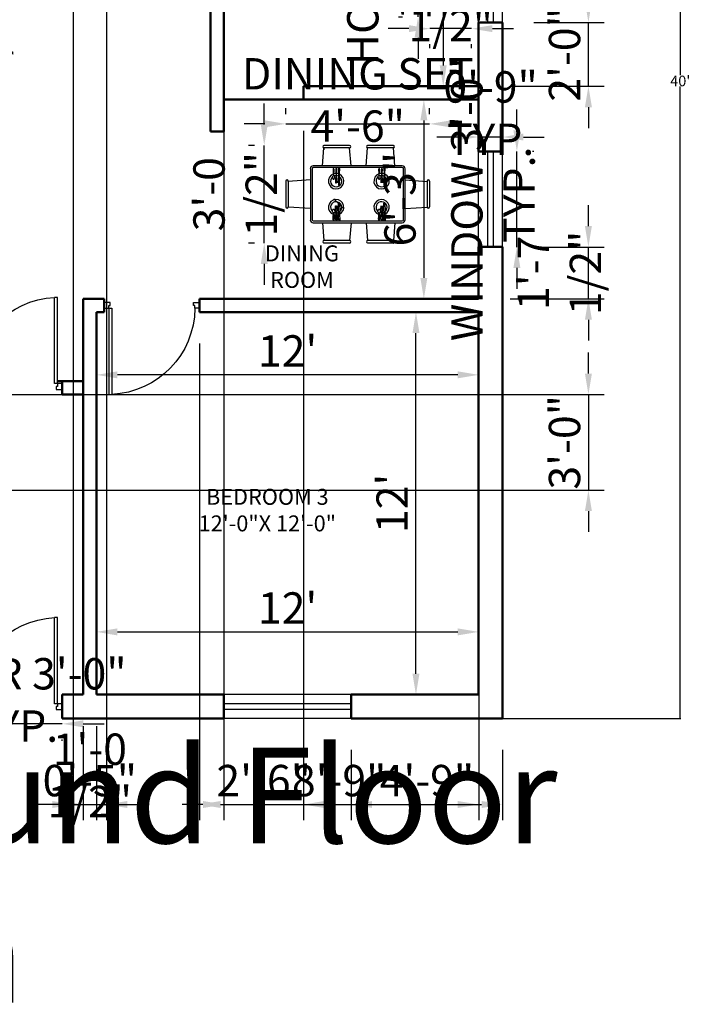
# Model space of a CAD drawing. Units: inches. Extents: x 117606 to 118050, y 251709 to 252357.
# Tile 2 of 3: x 117797 to 118050, y 251709 to 252079. Entities that reach past the tile are written whole.
import ezdxf

# ---------------------------------------------------------------- set-up
doc = ezdxf.new("R2010")
doc.units = ezdxf.units.IN
doc.header["$MEASUREMENT"] = 0
doc.layers.add('a patt', color=33, linetype='Continuous')
for name, color, linetype, lineweight in [('A-ANNO-TEXT', 7, 'Continuous', 25), ('A-AREA-IDEN', 7, 'Continuous', 25), ('A-DOOR', 4, 'Continuous', 25), ('FURNITURE', 53, 'Continuous', 18), ('WALL', 7, 'Continuous', 50), ('WINDOW', 2, 'Continuous', 25), ('YQ_DIM', 3, 'Continuous', 18)]:
    doc.layers.add(name, color=color, linetype=linetype, lineweight=lineweight)
doc.styles.get("Standard").update_dxf_attribs({"font": 'arial.ttf'})
doc.styles.add('YQ_DIM', font='SUPEROS.SHX', dxfattribs={"width": 0.8, "bigfont": 'HZDX.SHX'})
doc.dimstyles.get("Standard").update_dxf_attribs({"dimtxt": 4, "dimasz": 0.18, "dimexe": 0.18, "dimexo": 0.0625, "dimgap": 0.09, "dimtad": 0, "dimtih": 1, "dimtoh": 1, "dimzin": 0, "dimdsep": 46, "dimlunit": 4, "dimtxsty": 'Standard', "dimcen": 0.09, "dimadec": 0, "dimazin": 0, "dimtfac": 1, "dimtofl": 0, "dimtmove": 0, "dimatfit": 3, "dimfxl": 1, "dimtolj": 1, "dimtzin": 0, "dimarcsym": 0})
doc.dimstyles.new('yqi3_937', dxfattribs={"dimscale": 3.937008, "dimtxt": 3, "dimasz": 2, "dimexe": 1.5, "dimexo": 3, "dimgap": 0.5, "dimtad": 1, "dimdsep": 46, "dimlunit": 4, "dimtxsty": 'YQ_DIM', "dimcen": 0, "dimclrd": 256, "dimclre": 256, "dimclrt": 7, "dimadec": 1, "dimazin": 2, "dimtfac": 1, "dimtix": 1, "dimtmove": 2, "dimatfit": 2, "dimfxl": 1, "dimtolj": 1, "dimtzin": 0, "dimarcsym": 0})

# ---------------------------------------------------------------- blocks, each defined once
blk = doc.blocks.new('*D2')
at = {"layer": 'Defpoints', "color": 0, "transparency": 16777216}
for p in [(117978.89, 252296.28), (117978.89, 251816.28), (118045.85, 251816.28)]:
    blk.add_point(p, dxfattribs=at)
at = {"layer": 'YQ_DIM', "color": 0, "lineweight": -2, "transparency": 16777216}
for p, q in [((117978.95, 252296.28), (118046.03, 252296.28)), ((118045.85, 252296.1), (118045.85, 252058.42)), ((118045.85, 251816.46), (118045.85, 252054.15)), ((117978.95, 251816.28), (118046.03, 251816.28))]:
    blk.add_line(p, q, dxfattribs=at)
at = {"layer": 'YQ_DIM', "color": 0, "transparency": 16777216}
for points in [[(118045.82, 252296.1), (118045.88, 252296.1), (118045.85, 252296.28)], [(118045.82, 251816.46), (118045.88, 251816.46), (118045.85, 251816.28)]]:
    blk.add_solid(points, dxfattribs=at)
at = {"layer": 'YQ_DIM', "color": 0, "transparency": 16777216, "insert": (118045.85, 252056.28), "char_height": 4, "attachment_point": 5}
blk.add_mtext("\\A1;40'", dxfattribs=at)
blk = doc.blocks.new('*D6')
at = {"layer": 'Defpoints', "color": 0, "transparency": 16777216}
for p in [(117825.89, 251969.28), (117969.89, 251969.28), (117825.89, 251945.66)]:
    blk.add_point(p, dxfattribs=at)
at = {"layer": 'YQ_DIM', "color": 0, "lineweight": -2, "transparency": 16777216}
for p, q in [((117825.89, 251957.47), (117825.89, 251939.76)), ((117969.89, 251957.47), (117969.89, 251939.76)), ((117962.01, 251945.66), (117833.76, 251945.66))]:
    blk.add_line(p, q, dxfattribs=at)
at = {"layer": 'YQ_DIM', "color": 0, "transparency": 16777216}
for points in [[(117833.76, 251946.97), (117833.76, 251944.35), (117825.89, 251945.66)], [(117962.01, 251946.97), (117962.01, 251944.35), (117969.89, 251945.66)]]:
    blk.add_solid(points, dxfattribs=at)
at = {"layer": 'YQ_DIM', "color": 0, "transparency": 16777216, "insert": (117897.89, 251954.66), "char_height": 11.811, "attachment_point": 5, "style": 'YQ_DIM'}
blk.add_mtext("\\A1;12'", dxfattribs=at)
blk = doc.blocks.new('*D7')
at = {"layer": 'Defpoints', "color": 0, "transparency": 16777216}
for p in [(117969.89, 251848.91), (117825.89, 251825.28), (117969.89, 251825.28)]:
    blk.add_point(p, dxfattribs=at)
at = {"layer": 'YQ_DIM', "color": 0, "lineweight": -2, "transparency": 16777216}
for p, q in [((117825.89, 251837.1), (117825.89, 251854.81)), ((117969.89, 251837.1), (117969.89, 251854.81)), ((117833.76, 251848.91), (117962.01, 251848.91))]:
    blk.add_line(p, q, dxfattribs=at)
at = {"layer": 'YQ_DIM', "color": 0, "transparency": 16777216}
for points in [[(117833.76, 251850.22), (117833.76, 251847.59), (117825.89, 251848.91)], [(117962.01, 251850.22), (117962.01, 251847.59), (117969.89, 251848.91)]]:
    blk.add_solid(points, dxfattribs=at)
at = {"layer": 'YQ_DIM', "color": 0, "transparency": 16777216, "insert": (117897.89, 251857.9), "char_height": 11.811, "attachment_point": 5, "style": 'YQ_DIM'}
blk.add_mtext("\\A1;12'", dxfattribs=at)
blk = doc.blocks.new('*D8')
at = {"layer": 'Defpoints', "color": 0, "transparency": 16777216}
for p in [(117946.26, 251969.28), (117969.89, 251969.28), (117969.89, 251825.28)]:
    blk.add_point(p, dxfattribs=at)
at = {"layer": 'YQ_DIM', "color": 0, "lineweight": -2, "transparency": 16777216}
for p, q in [((117958.07, 251969.28), (117940.36, 251969.28)), ((117946.26, 251833.16), (117946.26, 251961.41)), ((117958.07, 251825.28), (117940.36, 251825.28))]:
    blk.add_line(p, q, dxfattribs=at)
at = {"layer": 'YQ_DIM', "color": 0, "transparency": 16777216}
for points in [[(117944.95, 251961.41), (117947.58, 251961.41), (117946.26, 251969.28)], [(117944.95, 251833.16), (117947.58, 251833.16), (117946.26, 251825.28)]]:
    blk.add_solid(points, dxfattribs=at)
at = {"layer": 'YQ_DIM', "color": 0, "transparency": 16777216, "insert": (117937.26, 251897.28), "char_height": 11.811, "attachment_point": 5, "rotation": 90, "style": 'YQ_DIM'}
blk.add_mtext("\\A1;12'", dxfattribs=at)
blk = doc.blocks.new('*D9')
at = {"layer": 'Defpoints', "color": 0, "transparency": 16777216}
for p in [(117969.89, 252138.28), (117956.53, 252054.28), (117969.89, 252054.28)]:
    blk.add_point(p, dxfattribs=at)
at = {"layer": 'YQ_DIM', "color": 0, "lineweight": -2, "transparency": 16777216}
for p, q in [((117958.07, 252138.28), (117950.63, 252138.28)), ((117956.53, 252130.41), (117956.53, 252062.16)), ((117958.07, 252054.28), (117950.63, 252054.28))]:
    blk.add_line(p, q, dxfattribs=at)
at = {"layer": 'YQ_DIM', "color": 0, "transparency": 16777216}
for points in [[(117955.22, 252130.41), (117957.84, 252130.41), (117956.53, 252138.28)], [(117955.22, 252062.16), (117957.84, 252062.16), (117956.53, 252054.28)]]:
    blk.add_solid(points, dxfattribs=at)
at = {"layer": 'YQ_DIM', "color": 0, "transparency": 16777216, "insert": (117947.53, 252096.28), "char_height": 11.811, "attachment_point": 5, "rotation": 90, "style": 'YQ_DIM'}
blk.add_mtext("\\A1;7'", dxfattribs=at)
blk = doc.blocks.new('*D10')
at = {"layer": 'Defpoints', "color": 0, "transparency": 16777216}
for p in [(117969.89, 252049.28), (117949.24, 251974.28), (117969.89, 251974.28)]:
    blk.add_point(p, dxfattribs=at)
at = {"layer": 'YQ_DIM', "color": 0, "lineweight": -2, "transparency": 16777216}
for p, q in [((117958.07, 252049.28), (117943.34, 252049.28)), ((117949.24, 252041.41), (117949.24, 251982.16)), ((117958.07, 251974.28), (117943.34, 251974.28))]:
    blk.add_line(p, q, dxfattribs=at)
at = {"layer": 'YQ_DIM', "color": 0, "transparency": 16777216}
for points in [[(117947.93, 252041.41), (117950.55, 252041.41), (117949.24, 252049.28)], [(117947.93, 251982.16), (117950.55, 251982.16), (117949.24, 251974.28)]]:
    blk.add_solid(points, dxfattribs=at)
at = {"layer": 'YQ_DIM', "color": 0, "transparency": 16777216, "insert": (117940.24, 252011.78), "char_height": 11.811, "attachment_point": 5, "rotation": 90, "style": 'YQ_DIM'}
blk.add_mtext('\\A1;6\'-3"', dxfattribs=at)
blk = doc.blocks.new('DR_D01')
for p, q in [((-0.45, 0.93), (-0.42, 0.93)), ((-0.45, 0.03), (-0.45, 0.93)), ((-0.42, 0.03), (-0.42, 0.93)), ((-0.5, 0.03), (-0.42, 0.03)), ((-0.5, 0.03), (-0.5, -0.03)), ((-0.45, 0.03), (-0.45, 0)), ((-0.45, 0), (-0.435, 0)), ((-0.435, 0), (-0.435, -0.03)), ((0.435, 0), (0.435, -0.03)), ((0.45, 0), (0.435, 0)), ((0.45, 0.03), (0.45, 0)), ((0.5, 0.03), (0.45, 0.03)), ((0.5, -0.03), (0.5, 0.03)), ((-0.435, -0.03), (-0.5, -0.03)), ((0.435, -0.03), (0.5, -0.03))]:
    blk.add_line(p, q)
blk.add_arc((-0.46, 0.021), 0.91, 0.5915, 87.4664)
blk = doc.blocks.new('WD_WIN4')
for p, q in [((-0.5, 0.5), (0.5, 0.5)), ((-0.5, 0.12), (0.5, 0.12)), ((-0.5, -0.12), (0.5, -0.12)), ((-0.5, -0.5), (0.5, -0.5))]:
    blk.add_line(p, q)
blk = doc.blocks.new('grdfg')
at = {"layer": 'a patt'}
for p, q in [((30493, 21433), (30516, 21715)), ((30514, 21715), (30514, 21683)), ((30519, 21754), (30516, 21754)), ((30923, 21715), (30516, 21715)), ((30920, 21754), (30519, 21754)), ((30519, 21754), (30519, 21754)), ((30920, 21754), (30923, 21754)), ((30946, 21433), (30923, 21715)), ((31186, 21433), (31208, 21715)), ((31615, 21715), (31208, 21715)), ((31212, 21754), (31209, 21754)), ((31212, 21754), (31212, 21754)), ((31612, 21754), (31212, 21754)), ((31612, 21754), (31615, 21754)), ((31638, 21433), (31615, 21715)), ((30509, 21606), (30507, 21606)), ((31202, 21606), (31200, 21606)), ((30302, 21386), (30302, 20580)), ((30329, 21386), (30329, 20580)), ((31755, 21433), (30348, 21433)), ((31755, 21405), (30348, 21405)), ((30745, 21374), (30767, 21374)), ((31464, 21374), (31486, 21374)), ((31774, 20580), (31774, 21386)), ((31802, 20580), (31802, 21386)), ((29914, 21190), (29914, 20783)), ((30302, 21212), (29953, 21187)), ((29953, 21187), (29953, 21190)), ((29953, 21187), (29953, 20786)), ((30667, 21293), (30673, 21293)), ((30667, 21284), (30673, 21284)), ((30717, 21262), (30710, 21262)), ((30710, 21250), (30717, 21250)), ((30749, 21275), (30763, 21275)), ((30749, 21264), (30763, 21264)), ((30749, 21257), (30763, 21257)), ((31386, 21293), (31392, 21293)), ((31386, 21284), (31392, 21284)), ((31436, 21262), (31429, 21262)), ((31429, 21250), (31436, 21250)), ((31468, 21275), (31482, 21275)), ((31468, 21264), (31482, 21264)), ((31468, 21257), (31482, 21257)), ((31802, 21212), (32150, 21187)), ((32150, 21187), (32150, 21190)), ((32150, 21187), (32150, 20786)), ((32189, 21190), (32189, 20783)), ((30674, 20910), (30827, 20756)), ((29953, 20786), (29953, 20783)), ((29953, 20786), (29953, 20786)), ((30302, 20760), (29953, 20780)), ((30710, 20716), (30717, 20716)), ((30717, 20704), (30710, 20704)), ((30749, 20709), (30763, 20709)), ((30749, 20702), (30763, 20702)), ((31429, 20716), (31436, 20716)), ((31436, 20704), (31429, 20704)), ((31468, 20709), (31482, 20709)), ((31468, 20702), (31482, 20702)), ((31802, 20760), (32150, 20780)), ((32150, 20786), (32150, 20786)), ((32150, 20786), (32150, 20783)), ((30348, 20561), (31755, 20561)), ((30667, 20682), (30673, 20682)), ((30667, 20673), (30673, 20673)), ((30675, 20640), (30707, 20640)), ((30720, 20640), (30748, 20640)), ((30745, 20592), (30767, 20592)), ((30749, 20691), (30763, 20691)), ((31386, 20682), (31392, 20682)), ((31386, 20673), (31392, 20673)), ((31394, 20640), (31426, 20640)), ((31439, 20640), (31467, 20640)), ((31464, 20592), (31486, 20592)), ((31468, 20691), (31482, 20691)), ((30348, 20533), (31755, 20533)), ((30493, 20533), (30516, 20251)), ((30946, 20533), (30923, 20251)), ((31186, 20533), (31208, 20251)), ((31638, 20533), (31615, 20251)), ((30509, 20360), (30507, 20360)), ((30514, 20283), (30514, 20251)), ((30923, 20251), (30516, 20251)), ((30932, 20360), (30930, 20360)), ((31615, 20251), (31208, 20251)), ((30519, 20212), (30516, 20212)), ((30920, 20212), (30519, 20212)), ((30519, 20212), (30519, 20212)), ((30920, 20212), (30923, 20212)), ((31212, 20212), (31209, 20212)), ((31212, 20212), (31212, 20212)), ((31612, 20212), (31212, 20212)), ((31612, 20212), (31615, 20212))]:
    blk.add_line(p, q, dxfattribs=at)
for points in [[(30663, 21372), (30663, 21360, -0.013852), (30667, 21293), (30667, 21284, -0.321801), (30662, 21276, 0.220637), (30653, 21261, 0.151079), (30660, 21225, 0.601255), (30681, 21225, 0.098298), (30689, 21251, 0.173345), (30683, 21272, 0.127575), (30676, 21278, -0.108886), (30673, 21284), (30673, 21293, -0.013852), (30678, 21360), (30678, 21372), (30676, 21387, 0.903848), (30664, 21387)], [(30745, 21391, 0.204141), (30745, 21374), (30749, 21319), (30749, 21275), (30747, 21267), (30749, 21264), (30749, 21257), (30747, 21251, -0.015744), (30745, 21126, 0.538165), (30763, 21126), (30769, 21251), (30763, 21257), (30763, 21264), (30765, 21267), (30763, 21275), (30763, 21319), (30767, 21374, 0.204141), (30767, 21391), (30762, 21392), (30751, 21392)], [(31382, 21372), (31382, 21360, -0.013852), (31386, 21293), (31386, 21284, -0.321801), (31381, 21276, 0.220637), (31372, 21261, 0.151079), (31379, 21225, 0.601255), (31400, 21225, 0.098298), (31408, 21251, 0.173345), (31402, 21272, 0.127575), (31395, 21278, -0.108886), (31392, 21284), (31392, 21293, -0.013852), (31397, 21360), (31397, 21372), (31395, 21387, 0.903848), (31383, 21387)], [(31464, 21391, 0.204141), (31464, 21374), (31468, 21319), (31468, 21275), (31466, 21267), (31468, 21264), (31468, 21257), (31466, 21251, -0.015744), (31464, 21126, 0.538165), (31482, 21126), (31488, 21251), (31482, 21257), (31482, 21264), (31484, 21267), (31482, 21275), (31482, 21319), (31486, 21374, 0.204141), (31486, 21391), (31481, 21392), (31470, 21392)], [(30663, 20594), (30663, 20606, 0.013852), (30667, 20673), (30667, 20682, 0.321801), (30662, 20690, -0.220637), (30653, 20705, -0.151079), (30660, 20741, -0.601255), (30681, 20741, -0.098298), (30689, 20715, -0.173345), (30683, 20694, -0.127575), (30676, 20688, 0.108886), (30673, 20682), (30673, 20673, 0.013852), (30678, 20606), (30678, 20594), (30676, 20579, -0.903848), (30664, 20579)], [(30745, 20575, -0.204141), (30745, 20592), (30749, 20647), (30749, 20691), (30747, 20699), (30749, 20702), (30749, 20709), (30747, 20715, 0.015744), (30745, 20840, -0.538165), (30763, 20840), (30769, 20715), (30763, 20709), (30763, 20702), (30765, 20699), (30763, 20691), (30763, 20647), (30767, 20592, -0.204141), (30767, 20575), (30762, 20574), (30751, 20574)], [(31382, 20594), (31382, 20606, 0.013852), (31386, 20673), (31386, 20682, 0.321801), (31381, 20690, -0.220637), (31372, 20705, -0.151079), (31379, 20741, -0.601255), (31400, 20741, -0.098298), (31408, 20715, -0.173345), (31402, 20694, -0.127575), (31395, 20688, 0.108886), (31392, 20682), (31392, 20673, 0.013852), (31397, 20606), (31397, 20594), (31395, 20579, -0.903848), (31383, 20579)], [(31464, 20575, -0.204141), (31464, 20592), (31468, 20647), (31468, 20691), (31466, 20699), (31468, 20702), (31468, 20709), (31466, 20715, 0.015744), (31464, 20840, -0.538165), (31482, 20840), (31488, 20715), (31482, 20709), (31482, 20702), (31484, 20699), (31482, 20691), (31482, 20647), (31486, 20592, -0.204141), (31486, 20575), (31481, 20574), (31470, 20574)]]:
    blk.add_lwpolyline(points, format="xyb", close=True, dxfattribs=at)
for points in [[(30706, 21387), (30704, 21369), (30704, 21355, -0.012883), (30710, 21262), (30710, 21250, -0.236068), (30703, 21239, 0.098033), (30699, 21219), (30701, 21164), (30703, 21164), (30704, 21219), (30706, 21219), (30708, 21164), (30710, 21164), (30712, 21221), (30713, 21223), (30715, 21221), (30717, 21164), (30719, 21164), (30720, 21219), (30722, 21219), (30724, 21164), (30726, 21164), (30728, 21219), (30724, 21239, -0.236068), (30717, 21250), (30717, 21262, -0.012883), (30722, 21355), (30722, 21369), (30720, 21387, 0.761905), (30706, 21387, 0.027392)], [(31425, 21387), (31423, 21369), (31423, 21355, -0.012883), (31429, 21262), (31429, 21250, -0.236068), (31422, 21239, 0.098033), (31418, 21219), (31420, 21164), (31422, 21164), (31423, 21219), (31425, 21219), (31427, 21164), (31429, 21164), (31431, 21221), (31432, 21223), (31434, 21221), (31436, 21164), (31438, 21164), (31439, 21219), (31441, 21219), (31443, 21164), (31445, 21164), (31447, 21219), (31443, 21239, -0.236068), (31436, 21250), (31436, 21262, -0.012883), (31441, 21355), (31441, 21369), (31439, 21387, 0.761905), (31425, 21387, 0.027392)], [(30706, 20579), (30704, 20597), (30704, 20611, 0.012883), (30710, 20704), (30710, 20716, 0.236068), (30703, 20727, -0.098033), (30699, 20747), (30701, 20802), (30703, 20802), (30704, 20747), (30706, 20747), (30708, 20802), (30710, 20802), (30712, 20745), (30713, 20743), (30715, 20745), (30717, 20802), (30719, 20802), (30720, 20747), (30722, 20747), (30724, 20802), (30726, 20802), (30728, 20747), (30724, 20727, 0.236068), (30717, 20716), (30717, 20704, 0.012883), (30722, 20611), (30722, 20597), (30720, 20579, -0.761905), (30706, 20579, -0.027392)], [(31425, 20579), (31423, 20597), (31423, 20611, 0.012883), (31429, 20704), (31429, 20716, 0.236068), (31422, 20727, -0.098033), (31418, 20747), (31420, 20802), (31422, 20802), (31423, 20747), (31425, 20747), (31427, 20802), (31429, 20802), (31431, 20745), (31432, 20743), (31434, 20745), (31436, 20802), (31438, 20802), (31439, 20747), (31441, 20747), (31443, 20802), (31445, 20802), (31447, 20747), (31443, 20727, 0.236068), (31436, 20716), (31436, 20704, 0.012883), (31441, 20611), (31441, 20597), (31439, 20579, -0.761905), (31425, 20579, -0.027392)]]:
    blk.add_lwpolyline(points, format="xyb", dxfattribs=at)
for centre, radius, start, end in [((30517, 21734), 19.5, 92.4912, 267.9051), ((30922, 21734), 19.5, 272.0949, 87.5088), ((31209, 21734), 19.5, 92.4912, 267.9051), ((31615, 21734), 19.5, 272.0949, 87.5088), ((30348, 21386), 46.6, 90, 180), ((30348, 21386), 18.7, 90, 180), ((31755, 21386), 46.6, 0, 90), ((31755, 21386), 18.7, 0, 90), ((29934, 21189), 19.5, 2.4912, 177.9051), ((30710, 21189), 122, 110.569, 64.0676), ((30710, 21189), 88.4, 130.4177, 52.8326), ((30710, 21189), 122, 91.1026, 107.1168), ((30710, 21189), 88.4, 90.4281, 108.0635), ((30710, 21189), 88.4, 64.8376, 85.191), ((30710, 21189), 122, 71.3681, 85.7295), ((31429, 21189), 122, 110.569, 64.0676), ((31429, 21189), 88.4, 130.4177, 52.8326), ((31429, 21189), 122, 91.1026, 107.1168), ((31429, 21189), 88.4, 90.4281, 108.0635), ((31429, 21189), 88.4, 64.8376, 85.191), ((31429, 21189), 122, 71.3681, 85.7295), ((32169, 21189), 19.5, 2.0949, 177.5088), ((30710, 20777), 122, 295.9324, 249.431), ((30710, 20777), 88.4, 307.1674, 229.5823), ((31429, 20777), 122, 295.9324, 249.431), ((31429, 20777), 88.4, 307.1674, 229.5823), ((29934, 20784), 19.5, 182.0949, 357.5088), ((30710, 20777), 88.4, 274.809, 295.1624), ((31429, 20777), 88.4, 274.809, 295.1624), ((32169, 20784), 19.5, 182.4912, 357.9051), ((30348, 20580), 46.6, 180, 270), ((30348, 20580), 18.7, 180, 270), ((30710, 20777), 122, 252.8832, 268.8974), ((30710, 20777), 88.4, 251.9365, 269.5719), ((30710, 20777), 122, 274.2705, 288.6319), ((31429, 20777), 122, 252.8832, 268.8974), ((31429, 20777), 88.4, 251.9365, 269.5719), ((31429, 20777), 122, 274.2705, 288.6319), ((31755, 20580), 46.6, 270, 0), ((31755, 20580), 18.7, 270, 0), ((30517, 20232), 19.5, 92.0949, 267.5088), ((30922, 20232), 19.5, 272.4912, 87.9051), ((31209, 20232), 19.5, 92.0949, 267.5088), ((31615, 20232), 19.5, 272.4912, 87.9051)]:
    blk.add_arc(centre, radius, start, end, dxfattribs=at)
blk = doc.blocks.new('*D143')
at = {"layer": 'Defpoints', "color": 0, "transparency": 16777216}
for p in [(117978.89, 252029.78), (117984.29, 252029.78), (117978.89, 251993.78)]:
    blk.add_point(p, dxfattribs=at)
at = {"layer": 'YQ_DIM', "lineweight": -2, "transparency": 16777216}
for p, q in [((117984.29, 252037.66), (117984.29, 252045.53)), ((117984.29, 251993.78), (117984.29, 252029.78)), ((117990.7, 252029.78), (117990.19, 252029.78)), ((117990.7, 251993.78), (117990.19, 251993.78)), ((117984.29, 251985.91), (117984.29, 251978.04))]:
    blk.add_line(p, q, dxfattribs=at)
at = {"layer": 'YQ_DIM', "transparency": 16777216}
for points in [[(117982.97, 252037.66), (117985.6, 252037.66), (117984.29, 252029.78)], [(117982.97, 251985.91), (117985.6, 251985.91), (117984.29, 251993.78)]]:
    blk.add_solid(points, dxfattribs=at)
at = {"layer": 'YQ_DIM', "color": 7, "transparency": 16777216, "insert": (117975.29, 252011.78), "char_height": 11.811, "attachment_point": 5, "rotation": 90, "style": 'YQ_DIM'}
blk.add_mtext('\\A1;WINDOW 3\'-0" TYP.', dxfattribs=at)
blk = doc.blocks.new('*D144')
at = {"layer": 'Defpoints', "color": 0, "transparency": 16777216}
for p in [(117969.89, 252035.18), (117969.89, 252029.78), (117978.89, 252029.78)]:
    blk.add_point(p, dxfattribs=at)
at = {"layer": 'YQ_DIM', "lineweight": -2, "transparency": 16777216}
for p, q in [((117969.89, 252041.6), (117969.89, 252041.09)), ((117978.89, 252041.6), (117978.89, 252041.09)), ((117962.01, 252035.18), (117954.14, 252035.18)), ((117978.89, 252035.18), (117969.89, 252035.18)), ((117986.76, 252035.18), (117994.63, 252035.18))]:
    blk.add_line(p, q, dxfattribs=at)
at = {"layer": 'YQ_DIM', "transparency": 16777216}
for points in [[(117962.01, 252036.5), (117962.01, 252033.87), (117969.89, 252035.18)], [(117986.76, 252036.5), (117986.76, 252033.87), (117978.89, 252035.18)]]:
    blk.add_solid(points, dxfattribs=at)
at = {"layer": 'YQ_DIM', "color": 7, "transparency": 16777216, "insert": (117974.39, 252044.18), "char_height": 11.811, "attachment_point": 5, "style": 'YQ_DIM'}
blk.add_mtext('\\A1;0\'-9" TYP.', dxfattribs=at)
blk = doc.blocks.new('*D147')
at = {"layer": 'Defpoints', "color": 0, "transparency": 16777216}
for p in [(117777.01, 251819.7), (117813.01, 251819.7), (117777.01, 251814.3)]:
    blk.add_point(p, dxfattribs=at)
at = {"layer": 'YQ_DIM', "lineweight": -2, "transparency": 16777216}
for p, q in [((117769.14, 251814.3), (117761.26, 251814.3)), ((117813.01, 251814.3), (117777.01, 251814.3)), ((117820.89, 251814.3), (117828.76, 251814.3)), ((117777.01, 251807.89), (117777.01, 251808.4)), ((117813.01, 251807.89), (117813.01, 251808.4))]:
    blk.add_line(p, q, dxfattribs=at)
at = {"layer": 'YQ_DIM', "transparency": 16777216}
for points in [[(117769.14, 251815.62), (117769.14, 251812.99), (117777.01, 251814.3)], [(117820.89, 251815.62), (117820.89, 251812.99), (117813.01, 251814.3)]]:
    blk.add_solid(points, dxfattribs=at)
at = {"layer": 'YQ_DIM', "color": 7, "transparency": 16777216, "insert": (117795.01, 251823.3), "char_height": 11.811, "attachment_point": 5, "style": 'YQ_DIM'}
blk.add_mtext('\\A1;DOOR 3\'-0" TYP.', dxfattribs=at)
blk = doc.blocks.new('*D153')
at = {"layer": 'Defpoints', "color": 0, "transparency": 16777216}
for p in [(117947.05, 252109.93), (117951.48, 252109.93), (117951.48, 252080.4)]:
    blk.add_point(p, dxfattribs=at)
at = {"layer": 'YQ_DIM', "lineweight": -2, "transparency": 16777216}
for p, q in [((117947.05, 252117.8), (117947.05, 252125.68)), ((117939.67, 252109.93), (117941.15, 252109.93)), ((117947.05, 252080.4), (117947.05, 252109.93)), ((117939.67, 252080.4), (117941.15, 252080.4)), ((117947.05, 252072.53), (117947.05, 252064.66))]:
    blk.add_line(p, q, dxfattribs=at)
at = {"layer": 'YQ_DIM', "transparency": 16777216}
for points in [[(117945.74, 252117.8), (117948.36, 252117.8), (117947.05, 252109.93)], [(117945.74, 252072.53), (117948.36, 252072.53), (117947.05, 252080.4)]]:
    blk.add_solid(points, dxfattribs=at)
at = {"layer": 'YQ_DIM', "color": 7, "transparency": 16777216, "insert": (117936.08, 252095.17), "char_height": 11.811, "attachment_point": 5, "rotation": 90, "style": 'YQ_DIM'}
blk.add_mtext('\\A1;HOB 2\'-5 1/2"', dxfattribs=at)
blk = doc.blocks.new('*D154')
at = {"layer": 'Defpoints', "color": 0, "transparency": 16777216}
for p in [(117951.48, 252080.4), (117967.23, 252080.4), (117951.48, 252075.97)]:
    blk.add_point(p, dxfattribs=at)
at = {"layer": 'YQ_DIM', "lineweight": -2, "transparency": 16777216}
for p, q in [((117943.61, 252075.97), (117935.73, 252075.97)), ((117967.23, 252075.97), (117951.48, 252075.97)), ((117975.1, 252075.97), (117982.98, 252075.97)), ((117951.48, 252068.59), (117951.48, 252070.07)), ((117967.23, 252068.59), (117967.23, 252070.07))]:
    blk.add_line(p, q, dxfattribs=at)
at = {"layer": 'YQ_DIM', "transparency": 16777216}
for points in [[(117943.61, 252077.29), (117943.61, 252074.66), (117951.48, 252075.97)], [(117975.1, 252077.29), (117975.1, 252074.66), (117967.23, 252075.97)]]:
    blk.add_solid(points, dxfattribs=at)
at = {"layer": 'YQ_DIM', "color": 7, "transparency": 16777216, "insert": (117959.36, 252086.94), "char_height": 11.811, "attachment_point": 5, "style": 'YQ_DIM'}
blk.add_mtext('\\A1;1\'-3 1/2"', dxfattribs=at)
blk = doc.blocks.new('*D157')
at = {"layer": 'Defpoints', "color": 0, "transparency": 16777216}
for p in [(117951.41, 252040.13), (117897.23, 252032), (117951.41, 252032)]:
    blk.add_point(p, dxfattribs=at)
at = {"layer": 'YQ_DIM', "lineweight": -2, "transparency": 16777216}
for p, q in [((117897.23, 252043.81), (117897.23, 252046.03)), ((117951.41, 252043.81), (117951.41, 252046.03)), ((117889.36, 252040.13), (117881.48, 252040.13)), ((117897.23, 252040.13), (117951.41, 252040.13)), ((117959.29, 252040.13), (117967.16, 252040.13))]:
    blk.add_line(p, q, dxfattribs=at)
at = {"layer": 'YQ_DIM', "transparency": 16777216}
for points in [[(117889.36, 252041.44), (117889.36, 252038.82), (117897.23, 252040.13)], [(117959.29, 252041.44), (117959.29, 252038.82), (117951.41, 252040.13)]]:
    blk.add_solid(points, dxfattribs=at)
at = {"layer": 'YQ_DIM', "color": 7, "transparency": 16777216, "insert": (117924.32, 252049.13), "char_height": 11.811, "attachment_point": 5, "style": 'YQ_DIM'}
blk.add_mtext('\\A1;DINING SET 4\'-6"', dxfattribs=at)
blk = doc.blocks.new('*D158')
at = {"layer": 'Defpoints', "color": 0, "transparency": 16777216}
for p in [(117889.1, 252032), (117897.23, 252032), (117897.23, 251995.28)]:
    blk.add_point(p, dxfattribs=at)
at = {"layer": 'YQ_DIM', "lineweight": -2, "transparency": 16777216}
for p, q in [((117889.1, 252039.88), (117889.1, 252047.75)), ((117885.42, 252032), (117883.2, 252032)), ((117889.1, 251995.28), (117889.1, 252032)), ((117885.42, 251995.28), (117883.2, 251995.28)), ((117889.1, 251987.4), (117889.1, 251979.53))]:
    blk.add_line(p, q, dxfattribs=at)
at = {"layer": 'YQ_DIM', "transparency": 16777216}
for points in [[(117887.79, 252039.88), (117890.41, 252039.88), (117889.1, 252032)], [(117887.79, 251987.4), (117890.41, 251987.4), (117889.1, 251995.28)]]:
    blk.add_solid(points, dxfattribs=at)
at = {"layer": 'YQ_DIM', "color": 7, "transparency": 16777216, "insert": (117878.13, 252013.64), "char_height": 11.811, "attachment_point": 5, "rotation": 90, "style": 'YQ_DIM'}
blk.add_mtext('\\A1;3\'-0 1/2"', dxfattribs=at)
blk = doc.blocks.new('*D159')
at = {"layer": 'Defpoints', "color": 0, "transparency": 16777216}
for p in [(117768.57, 252134.27), (117768.57, 252011.7), (117786.95, 252011.7)]:
    blk.add_point(p, dxfattribs=at)
at = {"layer": 'YQ_DIM', "lineweight": -2, "transparency": 16777216}
for p, q in [((117786.95, 252142.14), (117786.95, 252150.02)), ((117780.38, 252134.27), (117792.86, 252134.27)), ((117786.95, 252134.27), (117786.95, 252011.7)), ((117780.38, 252011.7), (117792.86, 252011.7)), ((117786.95, 252003.82), (117786.95, 251995.95))]:
    blk.add_line(p, q, dxfattribs=at)
at = {"layer": 'YQ_DIM', "transparency": 16777216}
for points in [[(117785.64, 252142.14), (117788.26, 252142.14), (117786.95, 252134.27)], [(117785.64, 252003.82), (117788.26, 252003.82), (117786.95, 252011.7)]]:
    blk.add_solid(points, dxfattribs=at)
at = {"layer": 'YQ_DIM', "color": 7, "transparency": 16777216, "insert": (117775.98, 252072.98), "char_height": 11.811, "attachment_point": 5, "rotation": 90, "style": 'YQ_DIM'}
blk.add_mtext('\\A1;SOFA SET 10\'-2 1/2"', dxfattribs=at)
blk = doc.blocks.new('*D169')
at = {"layer": 'Defpoints', "color": 0, "transparency": 16777216}
for p in [(117759.89, 251938.28), (117759.89, 251902.28), (118011.24, 251902.28)]:
    blk.add_point(p, dxfattribs=at)
at = {"layer": 'YQ_DIM', "lineweight": -2, "transparency": 16777216}
for p, q in [((118011.24, 251946.16), (118011.24, 251954.03)), ((117771.7, 251938.28), (118017.14, 251938.28)), ((118011.24, 251938.28), (118011.24, 251902.28)), ((117771.7, 251902.28), (118017.14, 251902.28)), ((118011.24, 251894.41), (118011.24, 251886.54))]:
    blk.add_line(p, q, dxfattribs=at)
at = {"layer": 'YQ_DIM', "transparency": 16777216}
for points in [[(118009.92, 251946.16), (118012.55, 251946.16), (118011.24, 251938.28)], [(118009.92, 251894.41), (118012.55, 251894.41), (118011.24, 251902.28)]]:
    blk.add_solid(points, dxfattribs=at)
at = {"layer": 'YQ_DIM', "color": 7, "transparency": 16777216, "insert": (118002.24, 251920.28), "char_height": 11.811, "attachment_point": 5, "rotation": 90, "style": 'YQ_DIM'}
blk.add_mtext('\\A1;3\'-0"', dxfattribs=at)
blk = doc.blocks.new('*D172')
at = {"layer": 'Defpoints', "color": 0, "transparency": 16777216}
for p in [(117921.89, 251816.28), (117978.89, 251816.28), (117978.89, 251783.93)]:
    blk.add_point(p, dxfattribs=at)
at = {"layer": 'YQ_DIM', "lineweight": -2, "transparency": 16777216}
for p, q in [((117921.89, 251804.47), (117921.89, 251778.03)), ((117978.89, 251804.47), (117978.89, 251778.03)), ((117929.76, 251783.93), (117971.01, 251783.93))]:
    blk.add_line(p, q, dxfattribs=at)
at = {"layer": 'YQ_DIM', "transparency": 16777216}
for points in [[(117929.76, 251785.25), (117929.76, 251782.62), (117921.89, 251783.93)], [(117971.01, 251785.25), (117971.01, 251782.62), (117978.89, 251783.93)]]:
    blk.add_solid(points, dxfattribs=at)
at = {"layer": 'YQ_DIM', "color": 7, "transparency": 16777216, "insert": (117950.39, 251792.93), "char_height": 11.811, "attachment_point": 5, "style": 'YQ_DIM'}
blk.add_mtext('\\A1;4\'-9"', dxfattribs=at)
blk = doc.blocks.new('*D174')
at = {"layer": 'Defpoints', "color": 0, "transparency": 16777216}
for p in [(117873.89, 252049.28), (117903.89, 252049.28), (117903.89, 251783.93)]:
    blk.add_point(p, dxfattribs=at)
at = {"layer": 'YQ_DIM', "lineweight": -2, "transparency": 16777216}
for p, q in [((117873.89, 252037.47), (117873.89, 251778.03)), ((117903.89, 252037.47), (117903.89, 251778.03)), ((117866.01, 251783.93), (117858.14, 251783.93)), ((117873.89, 251783.93), (117903.89, 251783.93)), ((117911.76, 251783.93), (117919.63, 251783.93))]:
    blk.add_line(p, q, dxfattribs=at)
at = {"layer": 'YQ_DIM', "transparency": 16777216}
for points in [[(117866.01, 251785.25), (117866.01, 251782.62), (117873.89, 251783.93)], [(117911.76, 251785.25), (117911.76, 251782.62), (117903.89, 251783.93)]]:
    blk.add_solid(points, dxfattribs=at)
at = {"layer": 'YQ_DIM', "color": 7, "transparency": 16777216, "insert": (117888.89, 251792.93), "char_height": 11.811, "attachment_point": 5, "style": 'YQ_DIM'}
blk.add_mtext('\\A1;2\'-6"', dxfattribs=at)
blk = doc.blocks.new('*D175')
at = {"layer": 'Defpoints', "color": 0, "transparency": 16777216}
for p in [(117820.89, 251825.28), (117825.89, 251825.28), (117825.89, 251783.93)]:
    blk.add_point(p, dxfattribs=at)
at = {"layer": 'YQ_DIM', "lineweight": -2, "transparency": 16777216}
for p, q in [((117820.89, 251813.47), (117820.89, 251778.03)), ((117825.89, 251813.47), (117825.89, 251778.03)), ((117813.01, 251783.93), (117805.14, 251783.93)), ((117820.89, 251783.93), (117825.89, 251783.93)), ((117833.76, 251783.93), (117841.63, 251783.93))]:
    blk.add_line(p, q, dxfattribs=at)
at = {"layer": 'YQ_DIM', "transparency": 16777216}
for points in [[(117813.01, 251785.25), (117813.01, 251782.62), (117820.89, 251783.93)], [(117833.76, 251785.25), (117833.76, 251782.62), (117825.89, 251783.93)]]:
    blk.add_solid(points, dxfattribs=at)
at = {"layer": 'YQ_DIM', "color": 7, "transparency": 16777216, "insert": (117823.39, 251792.93), "char_height": 11.811, "attachment_point": 5, "style": 'YQ_DIM'}
blk.add_mtext('\\A1;0\'-5"', dxfattribs=at)
blk = doc.blocks.new('*D178')
at = {"layer": 'Defpoints', "color": 0, "transparency": 16777216}
for p in [(117978.89, 251993.78), (118011.24, 251993.78), (117969.89, 251974.28)]:
    blk.add_point(p, dxfattribs=at)
at = {"layer": 'YQ_DIM', "lineweight": -2, "transparency": 16777216}
for p, q in [((118011.24, 252001.66), (118011.24, 252009.53)), ((117990.7, 251993.78), (118017.14, 251993.78)), ((118011.24, 251974.28), (118011.24, 251993.78)), ((117981.7, 251974.28), (118017.14, 251974.28)), ((118011.24, 251966.41), (118011.24, 251958.54))]:
    blk.add_line(p, q, dxfattribs=at)
at = {"layer": 'YQ_DIM', "transparency": 16777216}
for points in [[(118009.92, 252001.66), (118012.55, 252001.66), (118011.24, 251993.78)], [(118009.92, 251966.41), (118012.55, 251966.41), (118011.24, 251974.28)]]:
    blk.add_solid(points, dxfattribs=at)
at = {"layer": 'YQ_DIM', "color": 7, "transparency": 16777216, "insert": (118000.27, 251984.03), "char_height": 11.811, "attachment_point": 5, "rotation": 90, "style": 'YQ_DIM'}
blk.add_mtext('\\A1;1\'-7 1/2"', dxfattribs=at)
blk = doc.blocks.new('*D179')
at = {"layer": 'Defpoints', "color": 0, "transparency": 16777216}
for p in [(117978.89, 252078.28), (118011.24, 252078.28), (117969.89, 252054.28)]:
    blk.add_point(p, dxfattribs=at)
at = {"layer": 'YQ_DIM', "lineweight": -2, "transparency": 16777216}
for p, q in [((118011.24, 252086.16), (118011.24, 252094.03)), ((117990.7, 252078.28), (118017.14, 252078.28)), ((118011.24, 252054.28), (118011.24, 252078.28)), ((117981.7, 252054.28), (118017.14, 252054.28)), ((118011.24, 252046.41), (118011.24, 252038.54))]:
    blk.add_line(p, q, dxfattribs=at)
at = {"layer": 'YQ_DIM', "transparency": 16777216}
for points in [[(118009.92, 252086.16), (118012.55, 252086.16), (118011.24, 252078.28)], [(118009.92, 252046.41), (118012.55, 252046.41), (118011.24, 252054.28)]]:
    blk.add_solid(points, dxfattribs=at)
at = {"layer": 'YQ_DIM', "color": 7, "transparency": 16777216, "insert": (118002.24, 252066.28), "char_height": 11.811, "attachment_point": 5, "rotation": 90, "style": 'YQ_DIM'}
blk.add_mtext('\\A1;2\'-0"', dxfattribs=at)
blk = doc.blocks.new('*D181')
at = {"layer": 'Defpoints', "color": 0, "transparency": 16777216}
for p in [(117864.76, 251969.28), (117969.89, 251969.28), (117969.89, 251783.93)]:
    blk.add_point(p, dxfattribs=at)
at = {"layer": 'YQ_DIM', "lineweight": -2, "transparency": 16777216}
for p, q in [((117864.76, 251957.47), (117864.76, 251778.03)), ((117969.89, 251957.47), (117969.89, 251778.03)), ((117872.63, 251783.93), (117962.01, 251783.93))]:
    blk.add_line(p, q, dxfattribs=at)
at = {"layer": 'YQ_DIM', "transparency": 16777216}
for points in [[(117872.63, 251785.25), (117872.63, 251782.62), (117864.76, 251783.93)], [(117962.01, 251785.25), (117962.01, 251782.62), (117969.89, 251783.93)]]:
    blk.add_solid(points, dxfattribs=at)
at = {"layer": 'YQ_DIM', "color": 7, "transparency": 16777216, "insert": (117917.32, 251792.93), "char_height": 11.811, "attachment_point": 5, "style": 'YQ_DIM'}
blk.add_mtext('\\A1;8\'-9"', dxfattribs=at)
blk = doc.blocks.new('*D182')
at = {"layer": 'Defpoints', "color": 0, "transparency": 16777216}
for p in [(117817.14, 252143.28), (117829.63, 252143.28), (117829.63, 251783.93)]:
    blk.add_point(p, dxfattribs=at)
at = {"layer": 'YQ_DIM', "lineweight": -2, "transparency": 16777216}
for p, q in [((117817.14, 252131.47), (117817.14, 251778.03)), ((117829.63, 252131.47), (117829.63, 251778.03)), ((117809.26, 251783.93), (117801.39, 251783.93)), ((117817.14, 251783.93), (117829.63, 251783.93)), ((117837.51, 251783.93), (117845.38, 251783.93))]:
    blk.add_line(p, q, dxfattribs=at)
at = {"layer": 'YQ_DIM', "transparency": 16777216}
for points in [[(117809.26, 251785.25), (117809.26, 251782.62), (117817.14, 251783.93)], [(117837.51, 251785.25), (117837.51, 251782.62), (117829.63, 251783.93)]]:
    blk.add_solid(points, dxfattribs=at)
at = {"layer": 'YQ_DIM', "color": 7, "transparency": 16777216, "insert": (117823.39, 251794.9), "char_height": 11.811, "attachment_point": 5, "style": 'YQ_DIM'}
blk.add_mtext('\\A1;1\'-0 1/2"', dxfattribs=at)

msp = doc.modelspace()

# ---------------------------------------------------------------- linework, layer by layer
at = {"layer": 'WALL'}
for p, q in [((117868.885, 252049.284), (117868.885, 252138.284)), ((117873.885, 252054.284), (117873.885, 252138.284)), ((117969.885, 252029.784), (117969.885, 252078.284)), ((117969.885, 252078.284), (117978.885, 252078.284)), ((117978.885, 252029.784), (117978.885, 252078.284)), ((117873.885, 252054.284), (117873.885, 252049.284)), ((117903.885, 252054.284), (117969.885, 252054.284)), ((117903.885, 252054.284), (117903.885, 252049.284)), ((117868.885, 252037.284), (117868.885, 252049.284)), ((117873.885, 252049.284), (117969.885, 252049.284)), ((117873.885, 252049.284), (117873.885, 252037.284)), ((117873.885, 252037.284), (117868.885, 252037.284)), ((117969.885, 252029.784), (117978.885, 252029.784)), ((117969.885, 251974.284), (117969.885, 251993.784)), ((117969.885, 251993.784), (117978.885, 251993.784)), ((117978.885, 251816.284), (117978.885, 251993.784)), ((117820.885, 251825.284), (117820.885, 251974.284)), ((117820.885, 251974.284), (117828.759, 251974.284)), ((117828.759, 251974.284), (117828.759, 251969.284)), ((117864.759, 251974.284), (117868.885, 251974.284)), ((117864.759, 251974.284), (117864.759, 251969.284)), ((117868.885, 251974.284), (117969.885, 251974.284)), ((117825.885, 251825.284), (117825.885, 251969.284)), ((117825.885, 251969.284), (117828.759, 251969.284)), ((117864.759, 251969.284), (117969.885, 251969.284)), ((117969.885, 251825.284), (117969.885, 251969.284)), ((117820.885, 251943.284), (117811.211, 251943.284)), ((117813.011, 251943.259), (117813.011, 251938.259)), ((117820.885, 251938.284), (117813.011, 251938.284)), ((117813.011, 251825.284), (117820.885, 251825.284)), ((117813.011, 251825.284), (117813.011, 251816.284)), ((117825.885, 251825.284), (117873.885, 251825.284)), ((117873.885, 251825.284), (117873.885, 251816.284)), ((117921.885, 251825.284), (117969.885, 251825.284)), ((117921.885, 251825.284), (117921.885, 251816.284)), ((117813.011, 251816.284), (117873.885, 251816.284)), ((117921.885, 251816.284), (117978.885, 251816.284))]:
    msp.add_line(p, q, dxfattribs=at)

# ---------------------------------------------------------------- block references
at = {"layer": 'A-DOOR', "xscale": 36, "yscale": -36, "zscale": 36}
for p, rotation in [((117795.011, 251941.28), 180), ((117846.759, 251971.784), 4.63202e-11), ((117795.011, 251820.784), 180)]:
    msp.add_blockref('DR_D01', p, dxfattribs=dict(at, rotation=rotation))
at = {"layer": 'FURNITURE', "xscale": 0.0238200394065839, "yscale": 0.0238200394065839, "zscale": 0.0238200394065839}
msp.add_blockref('grdfg', (117184.672, 251513.824), dxfattribs=at)
at = {"layer": 'WINDOW'}
for p, xscale, yscale, zscale, rotation in [((117974.385, 252096.284), 36, 8.999999999985448, 36, 90), ((117974.385, 252011.784), 36, 8.999999999985448, 36, 90), ((117897.885, 251820.784), 48, 9.000000000029104, 48, 180.0000000000347)]:
    msp.add_blockref('WD_WIN4', p, dxfattribs=dict(at, xscale=xscale, yscale=yscale, zscale=zscale, rotation=rotation))

# ---------------------------------------------------------------- texts
at = {"layer": 'A-ANNO-TEXT', "insert": (117696.03, 251805.364), "char_height": 36, "width": 336.12923, "attachment_point": 1, "style": 'YQ_DIM'}
msp.add_mtext('Ground Floor Plan', dxfattribs=at)
at = {"layer": 'A-AREA-IDEN', "char_height": 6, "attachment_point": 1, "style": 'YQ_DIM'}
for s, insert, width in [('\\pxqc;DINING ROOM', (117883.318, 251994.393), 39.97217), ('\\pxqc;BEDROOM 3\\P12\'-0"X 12\'-0"', (117861.076, 251902.746), 58.36156)]:
    msp.add_mtext(s, dxfattribs=dict(at, insert=insert, width=width))

# ---------------------------------------------------------------- dimensions: what is measured, and where the dimension line sits
at = {"layer": 'YQ_DIM'}
for p1, p2, distance, dimstyle, picture, middle in [((117978.885, 252296.284), (117978.885, 251816.284), 66.964, 'Standard', '*D2', (118045.85, 252056.284)), ((117969.885, 252138.284), (117969.885, 252054.284), -13.355, 'yqi3_937', '*D9', (117947.532, 252096.284)), ((117969.885, 252049.284), (117969.885, 251974.284), -20.644, 'yqi3_937', '*D10', (117940.243, 252011.784))]:
    dim = msp.add_aligned_dim(p1=p1, p2=p2, distance=distance, dimstyle=dimstyle, override={"dimclrd": 0, "dimclre": 0, "dimclrt": 0}, dxfattribs=at)
    dim.commit()
    dim.dimension.update_dxf_attribs({"geometry": picture, "text_midpoint": middle})
for base, p1, p2, angle, text, picture, middle in [((117786.951, 252011.698), (117768.565, 252134.269), (117768.565, 252011.698), 270, 'SOFA SET <>', '*D159', (117775.983, 252072.983)), ((117947.052, 252109.931), (117951.481, 252080.403), (117951.481, 252109.931), 90, 'HOB <>', '*D153', (117936.085, 252095.167)), ((117984.285, 252029.784), (117978.885, 251993.784), (117978.885, 252029.784), 90, 'WINDOW <> TYP.', '*D143', (117975.287, 252011.784)), ((117969.885, 252035.184), (117978.885, 252029.784), (117969.885, 252029.784), 180, '<> TYP.', '*D144', (117974.385, 252044.183)), ((117777.011, 251814.304), (117813.011, 251819.704), (117777.011, 251819.704), 180, 'DOOR <> TYP.', '*D147', (117795.011, 251823.303))]:
    dim = msp.add_linear_dim(base=base, p1=p1, p2=p2, angle=angle, text=text, dimstyle='yqi3_937', override={"dimdec": 1, "dimlfac": 1, "dimrnd": 0, "dimzin": 1, "dimdsep": 46, "dimlunit": 4, "dimfrac": 2}, dxfattribs=at)
    dim.commit()
    dim.dimension.update_dxf_attribs({"geometry": picture, "text_midpoint": middle})
for base, p1, p2, override, picture, middle in [((117829.633, 251783.934), (117817.137, 252143.284), (117829.633, 252143.279), {"dimdec": 1, "dimlfac": 1, "dimrnd": 0, "dimzin": 1, "dimdsep": 46, "dimlunit": 4, "dimfrac": 2}, '*D182', (117823.385, 251794.901)), ((117903.885, 251783.934), (117873.885, 252049.284), (117903.885, 252049.284), {"dimdec": 1, "dimlfac": 1, "dimrnd": 0, "dimzin": 1, "dimdsep": 46, "dimlunit": 4, "dimfrac": 2}, '*D174', (117888.885, 251792.933)), ((117969.885, 251783.934), (117864.759, 251969.284), (117969.885, 251969.284), {"dimdec": 1, "dimlfac": 1, "dimrnd": 0, "dimzin": 1, "dimdsep": 46, "dimlunit": 4, "dimfrac": 2}, '*D181', (117917.322, 251792.933)), ((117969.885, 251848.906), (117825.885, 251825.284), (117969.885, 251825.284), {"dimclrd": 0, "dimclre": 0, "dimclrt": 0}, '*D7', (117897.885, 251857.905)), ((117825.885, 251783.934), (117820.885, 251825.284), (117825.885, 251825.284), {"dimdec": 1, "dimlfac": 1, "dimrnd": 0, "dimzin": 1, "dimdsep": 46, "dimlunit": 4, "dimfrac": 2}, '*D175', (117823.385, 251792.933)), ((117978.885, 251783.934), (117921.885, 251816.284), (117978.885, 251816.284), {"dimdec": 1, "dimlfac": 1, "dimrnd": 0, "dimzin": 1, "dimdsep": 46, "dimlunit": 4, "dimfrac": 2}, '*D172', (117950.385, 251792.933))]:
    dim = msp.add_linear_dim(base=base, p1=p1, p2=p2, dimstyle='yqi3_937', override=override, dxfattribs=at)
    dim.commit()
    dim.dimension.update_dxf_attribs({"geometry": picture, "text_midpoint": middle})
for base, p1, p2, angle, override, picture, middle in [((117951.481, 252075.974), (117967.229, 252080.403), (117951.481, 252080.403), 180, {"dimdec": 1, "dimlfac": 1, "dimrnd": 0, "dimzin": 1, "dimdsep": 46, "dimlunit": 4, "dimfrac": 2}, '*D154', (117959.355, 252086.941)), ((118011.235, 252078.284), (117969.885, 252054.284), (117978.885, 252078.284), 90, {"dimdec": 1, "dimlfac": 1, "dimrnd": 0, "dimzin": 1, "dimdsep": 46, "dimlunit": 4, "dimfrac": 2}, '*D179', (118002.237, 252066.284)), ((117889.102, 252032.002), (117897.23, 251995.278), (117897.23, 252032.002), 90, {"dimdec": 1, "dimlfac": 1, "dimrnd": 0, "dimzin": 1, "dimdsep": 46, "dimlunit": 4, "dimfrac": 2}, '*D158', (117878.135, 252013.64)), ((118011.235, 251993.784), (117969.885, 251974.284), (117978.885, 251993.784), 90, {"dimdec": 1, "dimlfac": 1, "dimrnd": 0, "dimzin": 1, "dimdsep": 46, "dimlunit": 4, "dimfrac": 2}, '*D178', (118000.268, 251984.034)), ((117825.885, 251945.662), (117969.885, 251969.284), (117825.885, 251969.284), 180, {"dimclrd": 0, "dimclre": 0, "dimclrt": 0}, '*D6', (117897.885, 251954.661)), ((117946.263, 251969.284), (117969.885, 251825.284), (117969.885, 251969.284), 90, {"dimclrd": 0, "dimclre": 0, "dimclrt": 0}, '*D8', (117937.264, 251897.284)), ((118011.235, 251902.284), (117759.885, 251938.284), (117759.885, 251902.284), 90, {"dimdec": 1, "dimlfac": 1, "dimrnd": 0, "dimzin": 1, "dimdsep": 46, "dimlunit": 4, "dimfrac": 2}, '*D169', (118002.237, 251920.284))]:
    dim = msp.add_linear_dim(base=base, p1=p1, p2=p2, angle=angle, dimstyle='yqi3_937', override=override, dxfattribs=at)
    dim.commit()
    dim.dimension.update_dxf_attribs({"geometry": picture, "text_midpoint": middle})
dim = msp.add_linear_dim(base=(117951.412, 252040.129), p1=(117897.23, 252032.002), p2=(117951.412, 252032.002), text='DINING SET <>', dimstyle='yqi3_937', override={"dimdec": 1, "dimlfac": 1, "dimrnd": 0, "dimzin": 1, "dimdsep": 46, "dimlunit": 4, "dimfrac": 2}, dxfattribs=at)
dim.commit()
dim.dimension.update_dxf_attribs({"geometry": '*D157', "text_midpoint": (117924.321, 252049.128)})

doc.saveas('drawing.dxf')
